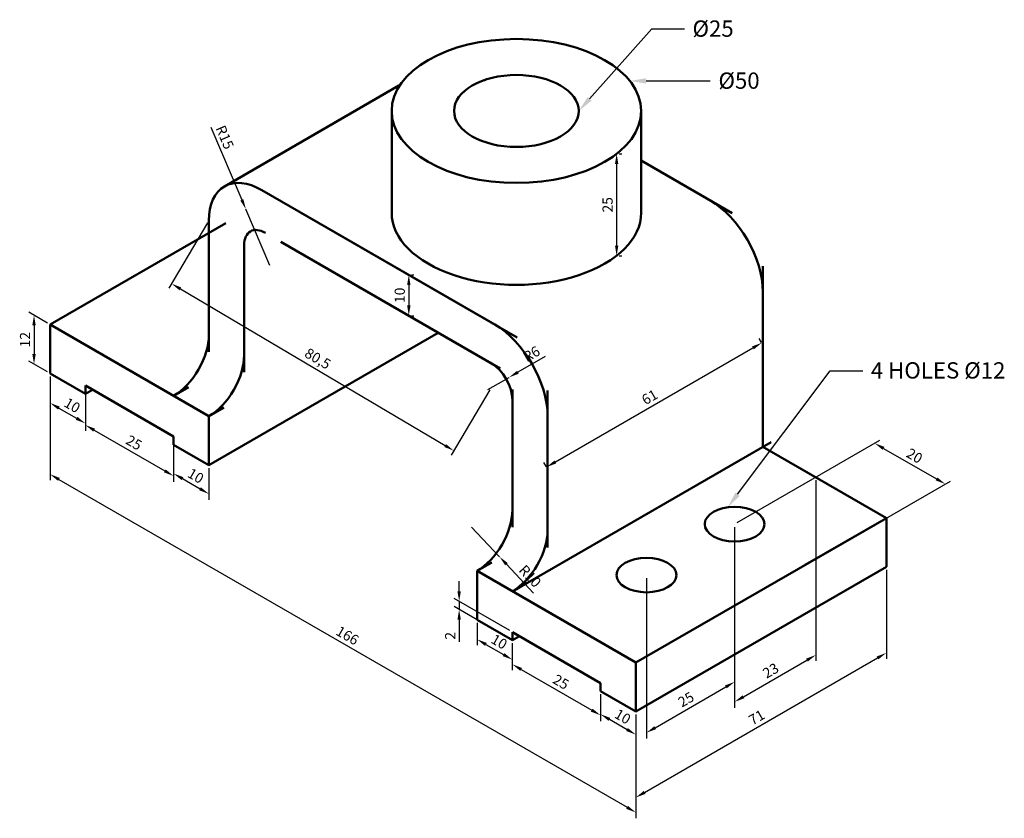
# Model space of a CAD drawing. Units: millimetres. Extents: x 2147 to 2389, y 1166 to 1362.
import ezdxf
from ezdxf import colors
from ezdxf.entities.mleader import LeaderData, LeaderLine
from ezdxf.math import Vec2, Vec3

# ---------------------------------------------------------------- set-up
doc = ezdxf.new("R2010")
doc.units = ezdxf.units.MM
for name, color, linetype, lineweight in [('M-DIMS', 2, 'Continuous', 25), ('M-OUTL', 7, 'Continuous', 50), ('M-TEXT', 3, 'Continuous', 25)]:
    doc.layers.add(name, color=color, linetype=linetype, lineweight=lineweight)
doc.styles.get("Standard").update_dxf_attribs({"font": 'arial.ttf'})
doc.dimstyles.new('ISO-25', dxfattribs={"dimtxt": 2.5, "dimasz": 2.5, "dimexe": 1.25, "dimexo": 0.625, "dimtad": 1, "dimtxsty": 'Standard', "dimcen": 2.5, "dimadec": 0, "dimazin": 0, "dimtfac": 1, "dimtmove": 0, "dimatfit": 3, "dimfxl": 1, "dimarcsym": 0})

# ---------------------------------------------------------------- blocks, each defined once
blk = doc.blocks.new('*D1')
at = {"layer": 'Defpoints', "color": 0, "transparency": 16777216}
for p in [(2154.59, 1274.83), (2298.35, 1191.83), (2298.35, 1167.06)]:
    blk.add_point(p, dxfattribs=at)
at = {"layer": 'M-DIMS', "color": 0, "lineweight": -2, "transparency": 16777216}
for p, q in [((2154.59, 1274.1), (2154.59, 1248.61)), ((2156.76, 1248.81), (2296.19, 1168.31)), ((2298.35, 1191.1), (2298.35, 1165.61))]:
    blk.add_line(p, q, dxfattribs=at)
at = {"layer": 'M-DIMS', "color": 0, "transparency": 16777216}
for points in [[(2156.97, 1249.17), (2156.55, 1248.44), (2154.59, 1250.06)], [(2296.4, 1168.67), (2295.98, 1167.94), (2298.35, 1167.06)]]:
    blk.add_solid(points, dxfattribs=at)
at = {"layer": 'M-DIMS', "color": 0, "transparency": 16777216, "insert": (2227.42, 1210.2), "char_height": 2.5, "attachment_point": 5, "rotation": 330}
blk.add_mtext('166', dxfattribs=at)
blk = doc.blocks.new('*D2')
at = {"layer": 'Defpoints', "color": 0, "transparency": 16777216}
for p in [(2154.59, 1274.83), (2163.25, 1269.83), (2163.25, 1262.56)]:
    blk.add_point(p, dxfattribs=at)
at = {"layer": 'M-DIMS', "color": 0, "lineweight": -2, "transparency": 16777216}
for p, q in [((2154.59, 1274.1), (2154.59, 1266.12)), ((2163.25, 1269.1), (2163.25, 1261.12)), ((2156.76, 1266.31), (2161.09, 1263.81))]:
    blk.add_line(p, q, dxfattribs=at)
at = {"layer": 'M-DIMS', "color": 0, "transparency": 16777216}
for points in [[(2156.97, 1266.67), (2156.55, 1265.95), (2154.59, 1267.56)], [(2161.3, 1264.17), (2160.88, 1263.45), (2163.25, 1262.56)]]:
    blk.add_solid(points, dxfattribs=at)
at = {"layer": 'M-DIMS', "color": 0, "transparency": 16777216, "insert": (2159.87, 1266.71), "char_height": 2.5, "attachment_point": 5, "rotation": 330}
blk.add_mtext('10', dxfattribs=at)
blk = doc.blocks.new('*D3')
at = {"layer": 'Defpoints', "color": 0, "transparency": 16777216}
for p in [(2163.25, 1271.83), (2184.9, 1259.33), (2184.9, 1249.65)]:
    blk.add_point(p, dxfattribs=at)
at = {"layer": 'M-DIMS', "color": 0, "lineweight": -2, "transparency": 16777216}
for p, q in [((2163.25, 1271.1), (2163.25, 1260.71)), ((2165.42, 1260.9), (2182.74, 1250.9)), ((2184.9, 1258.6), (2184.9, 1248.21))]:
    blk.add_line(p, q, dxfattribs=at)
at = {"layer": 'M-DIMS', "color": 0, "transparency": 16777216}
for points in [[(2165.63, 1261.26), (2165.21, 1260.54), (2163.25, 1262.15)], [(2182.95, 1251.26), (2182.53, 1250.54), (2184.9, 1249.65)]]:
    blk.add_solid(points, dxfattribs=at)
at = {"layer": 'M-DIMS', "color": 0, "transparency": 16777216, "insert": (2175.03, 1257.55), "char_height": 2.5, "attachment_point": 5, "rotation": 330}
blk.add_mtext('25', dxfattribs=at)
blk = doc.blocks.new('*D4')
at = {"layer": 'Defpoints', "color": 0, "transparency": 16777216}
for p in [(2184.9, 1257.33), (2193.56, 1252.33), (2193.56, 1245.25)]:
    blk.add_point(p, dxfattribs=at)
at = {"layer": 'M-DIMS', "color": 0, "lineweight": -2, "transparency": 16777216}
for p, q in [((2184.9, 1256.6), (2184.9, 1248.81)), ((2193.56, 1251.6), (2193.56, 1243.81)), ((2187.07, 1249), (2191.4, 1246.5))]:
    blk.add_line(p, q, dxfattribs=at)
at = {"layer": 'M-DIMS', "color": 0, "transparency": 16777216}
for points in [[(2187.28, 1249.36), (2186.86, 1248.64), (2184.9, 1250.25)], [(2191.61, 1246.86), (2191.19, 1246.14), (2193.56, 1245.25)]]:
    blk.add_solid(points, dxfattribs=at)
at = {"layer": 'M-DIMS', "color": 0, "transparency": 16777216, "insert": (2190.18, 1249.4), "char_height": 2.5, "attachment_point": 5, "rotation": 330}
blk.add_mtext('10', dxfattribs=at)
blk = doc.blocks.new('*D5')
at = {"layer": 'Defpoints', "color": 0, "transparency": 16777216}
for p in [(2154.59, 1286.83), (2150.65, 1277.1), (2154.59, 1274.83)]:
    blk.add_point(p, dxfattribs=at)
at = {"layer": 'M-DIMS', "color": 0, "lineweight": -2, "transparency": 16777216}
for p, q in [((2153.97, 1287.19), (2149.4, 1289.82)), ((2150.65, 1286.6), (2150.65, 1279.6)), ((2153.97, 1275.19), (2149.4, 1277.82))]:
    blk.add_line(p, q, dxfattribs=at)
at = {"layer": 'M-DIMS', "color": 0, "transparency": 16777216}
for points in [[(2150.23, 1286.6), (2151.07, 1286.6), (2150.65, 1289.1)], [(2150.23, 1279.6), (2151.07, 1279.6), (2150.65, 1277.1)]]:
    blk.add_solid(points, dxfattribs=at)
at = {"layer": 'M-DIMS', "color": 0, "transparency": 16777216, "insert": (2148.77, 1283.1), "char_height": 2.5, "attachment_point": 5, "rotation": 90}
blk.add_mtext('12', dxfattribs=at)
blk = doc.blocks.new('*D6')
at = {"layer": 'Defpoints', "color": 0, "transparency": 16777216}
for p in [(2259.38, 1214.33), (2268.04, 1209.33), (2268.04, 1204.55)]:
    blk.add_point(p, dxfattribs=at)
at = {"layer": 'M-DIMS', "color": 0, "lineweight": -2, "transparency": 16777216}
for p, q in [((2259.38, 1213.6), (2259.38, 1208.1)), ((2268.04, 1208.6), (2268.04, 1203.1)), ((2261.55, 1208.3), (2265.88, 1205.8))]:
    blk.add_line(p, q, dxfattribs=at)
at = {"layer": 'M-DIMS', "color": 0, "transparency": 16777216}
for points in [[(2261.76, 1208.66), (2261.34, 1207.94), (2259.38, 1209.55)], [(2266.09, 1206.16), (2265.67, 1205.44), (2268.04, 1204.55)]]:
    blk.add_solid(points, dxfattribs=at)
at = {"layer": 'M-DIMS', "color": 0, "transparency": 16777216, "insert": (2264.66, 1208.69), "char_height": 2.5, "attachment_point": 5, "rotation": 330}
blk.add_mtext('10', dxfattribs=at)
blk = doc.blocks.new('*D7')
at = {"layer": 'Defpoints', "color": 0, "transparency": 16777216}
for p in [(2254.99, 1216.86), (2268.04, 1211.33), (2268.04, 1209.33)]:
    blk.add_point(p, dxfattribs=at)
at = {"layer": 'M-DIMS', "color": 0, "lineweight": -2, "transparency": 16777216}
for p, q in [((2254.99, 1221.36), (2254.99, 1223.86)), ((2267.42, 1211.69), (2253.74, 1219.59)), ((2254.99, 1218.86), (2254.99, 1216.86)), ((2267.42, 1209.69), (2253.74, 1217.59)), ((2254.99, 1214.36), (2254.99, 1208.96))]:
    blk.add_line(p, q, dxfattribs=at)
at = {"layer": 'M-DIMS', "color": 0, "transparency": 16777216}
for points in [[(2254.57, 1221.36), (2255.4, 1221.36), (2254.99, 1218.86)], [(2254.57, 1214.36), (2255.4, 1214.36), (2254.99, 1216.86)]]:
    blk.add_solid(points, dxfattribs=at)
at = {"layer": 'M-DIMS', "color": 0, "transparency": 16777216, "insert": (2253.11, 1210.41), "char_height": 2.5, "attachment_point": 5, "rotation": 90}
blk.add_mtext('2', dxfattribs=at)
blk = doc.blocks.new('*D8')
at = {"layer": 'Defpoints', "color": 0, "transparency": 16777216}
for p in [(2268.04, 1209.33), (2289.69, 1196.83), (2289.69, 1190.91)]:
    blk.add_point(p, dxfattribs=at)
at = {"layer": 'M-DIMS', "color": 0, "lineweight": -2, "transparency": 16777216}
for p, q in [((2268.04, 1208.6), (2268.04, 1201.97)), ((2270.21, 1202.16), (2287.53, 1192.16)), ((2289.69, 1196.1), (2289.69, 1189.47))]:
    blk.add_line(p, q, dxfattribs=at)
at = {"layer": 'M-DIMS', "color": 0, "transparency": 16777216}
for points in [[(2270.42, 1202.52), (2270, 1201.8), (2268.04, 1203.41)], [(2287.74, 1192.52), (2287.32, 1191.8), (2289.69, 1190.91)]]:
    blk.add_solid(points, dxfattribs=at)
at = {"layer": 'M-DIMS', "color": 0, "transparency": 16777216, "insert": (2279.82, 1198.81), "char_height": 2.5, "attachment_point": 5, "rotation": 330}
blk.add_mtext('25', dxfattribs=at)
blk = doc.blocks.new('*D9')
at = {"layer": 'Defpoints', "color": 0, "transparency": 16777216}
for p in [(2289.69, 1196.83), (2298.35, 1191.83), (2298.35, 1186.16)]:
    blk.add_point(p, dxfattribs=at)
at = {"layer": 'M-DIMS', "color": 0, "lineweight": -2, "transparency": 16777216}
for p, q in [((2289.69, 1196.1), (2289.69, 1189.72)), ((2291.86, 1189.91), (2296.19, 1187.41)), ((2298.35, 1191.1), (2298.35, 1184.72))]:
    blk.add_line(p, q, dxfattribs=at)
at = {"layer": 'M-DIMS', "color": 0, "transparency": 16777216}
for points in [[(2292.07, 1190.27), (2291.65, 1189.55), (2289.69, 1191.16)], [(2296.4, 1187.77), (2295.98, 1187.05), (2298.35, 1186.16)]]:
    blk.add_solid(points, dxfattribs=at)
at = {"layer": 'M-DIMS', "color": 0, "transparency": 16777216, "insert": (2294.97, 1190.31), "char_height": 2.5, "attachment_point": 5, "rotation": 330}
blk.add_mtext('10', dxfattribs=at)
blk = doc.blocks.new('*D10')
at = {"layer": 'Defpoints', "color": 0, "transparency": 16777216}
for p in [(2359.84, 1227.33), (2359.84, 1206.23), (2298.35, 1191.83)]:
    blk.add_point(p, dxfattribs=at)
at = {"layer": 'M-DIMS', "color": 0, "lineweight": -2, "transparency": 16777216}
for p, q in [((2359.84, 1226.6), (2359.84, 1204.79)), ((2300.52, 1171.98), (2357.68, 1204.98)), ((2298.35, 1191.1), (2298.35, 1169.29))]:
    blk.add_line(p, q, dxfattribs=at)
at = {"layer": 'M-DIMS', "color": 0, "transparency": 16777216}
for points in [[(2357.47, 1205.34), (2357.88, 1204.62), (2359.84, 1206.23)], [(2300.31, 1172.34), (2300.73, 1171.62), (2298.35, 1170.73)]]:
    blk.add_solid(points, dxfattribs=at)
at = {"layer": 'M-DIMS', "color": 0, "transparency": 16777216, "insert": (2328.16, 1190.11), "char_height": 2.5, "attachment_point": 5, "rotation": 30}
blk.add_mtext('71', dxfattribs=at)
blk = doc.blocks.new('*D11')
at = {"layer": 'Defpoints', "color": 0, "transparency": 16777216}
for p in [(2322.6, 1237.83), (2300.95, 1225.33), (2322.6, 1199.11)]:
    blk.add_point(p, dxfattribs=at)
at = {"layer": 'M-DIMS', "color": 0, "lineweight": -2, "transparency": 16777216}
for p, q in [((2322.6, 1237.1), (2322.6, 1197.67)), ((2300.95, 1224.6), (2300.95, 1185.17)), ((2303.12, 1187.86), (2320.44, 1197.86))]:
    blk.add_line(p, q, dxfattribs=at)
at = {"layer": 'M-DIMS', "color": 0, "transparency": 16777216}
for points in [[(2320.23, 1198.22), (2320.65, 1197.5), (2322.6, 1199.11)], [(2302.91, 1188.22), (2303.32, 1187.5), (2300.95, 1186.61)]]:
    blk.add_solid(points, dxfattribs=at)
at = {"layer": 'M-DIMS', "color": 0, "transparency": 16777216, "insert": (2310.83, 1194.51), "char_height": 2.5, "attachment_point": 5, "rotation": 30}
blk.add_mtext('25', dxfattribs=at)
blk = doc.blocks.new('*D12')
at = {"layer": 'Defpoints', "color": 0, "transparency": 16777216}
for p in [(2374.31, 1247.68), (2322.6, 1237.83), (2339.92, 1227.83)]:
    blk.add_point(p, dxfattribs=at)
at = {"layer": 'M-DIMS', "color": 0, "lineweight": -2, "transparency": 16777216}
for p, q in [((2323.23, 1238.19), (2358.23, 1258.4)), ((2359.15, 1256.43), (2372.14, 1248.93)), ((2340.55, 1228.19), (2375.56, 1248.4))]:
    blk.add_line(p, q, dxfattribs=at)
at = {"layer": 'M-DIMS', "color": 0, "transparency": 16777216}
for points in [[(2359.36, 1256.79), (2358.94, 1256.07), (2356.98, 1257.68)], [(2372.35, 1249.29), (2371.93, 1248.57), (2374.31, 1247.68)]]:
    blk.add_solid(points, dxfattribs=at)
at = {"layer": 'M-DIMS', "color": 0, "transparency": 16777216, "insert": (2366.6, 1254.32), "char_height": 2.5, "attachment_point": 5, "rotation": 330}
blk.add_mtext('20', dxfattribs=at)
blk = doc.blocks.new('*D13')
at = {"layer": 'Defpoints', "color": 0, "transparency": 16777216}
for p in [(2242.63, 1299), (2242.63, 1289), (2242.63, 1289)]:
    blk.add_point(p, dxfattribs=at)
at = {"layer": 'M-DIMS', "color": 0, "lineweight": -2, "transparency": 16777216}
for p, q in [((2243.26, 1299), (2243.88, 1299)), ((2242.63, 1296.5), (2242.63, 1291.5)), ((2243.26, 1289), (2243.88, 1289))]:
    blk.add_line(p, q, dxfattribs=at)
at = {"layer": 'M-DIMS', "color": 0, "transparency": 16777216}
for points in [[(2242.22, 1296.5), (2243.05, 1296.5), (2242.63, 1299)], [(2242.22, 1291.5), (2243.05, 1291.5), (2242.63, 1289)]]:
    blk.add_solid(points, dxfattribs=at)
at = {"layer": 'M-DIMS', "color": 0, "transparency": 16777216, "insert": (2240.73, 1294), "char_height": 2.5, "attachment_point": 5, "rotation": 90}
blk.add_mtext('10', dxfattribs=at)
blk = doc.blocks.new('*D14')
at = {"layer": 'Defpoints', "color": 0, "transparency": 16777216}
for p in [(2293.64, 1328.72), (2293.64, 1303.72), (2293.64, 1303.72)]:
    blk.add_point(p, dxfattribs=at)
at = {"layer": 'M-DIMS', "color": 0, "lineweight": -2, "transparency": 16777216}
for p, q in [((2294.27, 1328.72), (2294.89, 1328.72)), ((2293.64, 1326.22), (2293.64, 1306.22)), ((2294.27, 1303.72), (2294.89, 1303.72))]:
    blk.add_line(p, q, dxfattribs=at)
at = {"layer": 'M-DIMS', "color": 0, "transparency": 16777216}
for points in [[(2293.23, 1326.22), (2294.06, 1326.22), (2293.64, 1328.72)], [(2293.23, 1306.22), (2294.06, 1306.22), (2293.64, 1303.72)]]:
    blk.add_solid(points, dxfattribs=at)
at = {"layer": 'M-DIMS', "color": 0, "transparency": 16777216, "insert": (2291.74, 1316.22), "char_height": 2.5, "attachment_point": 5, "rotation": 90}
blk.add_mtext('25', dxfattribs=at)
blk = doc.blocks.new('*D15')
at = {"layer": 'Defpoints', "color": 0, "transparency": 16777216}
for p in [(2342.52, 1249.33), (2322.6, 1237.83), (2342.52, 1205.7)]:
    blk.add_point(p, dxfattribs=at)
at = {"layer": 'M-DIMS', "color": 0, "lineweight": -2, "transparency": 16777216}
for p, q in [((2342.52, 1248.6), (2342.52, 1204.25)), ((2322.6, 1237.1), (2322.6, 1192.75)), ((2324.77, 1195.45), (2340.36, 1204.45))]:
    blk.add_line(p, q, dxfattribs=at)
at = {"layer": 'M-DIMS', "color": 0, "transparency": 16777216}
for points in [[(2340.15, 1204.81), (2340.56, 1204.08), (2342.52, 1205.7)], [(2324.56, 1195.81), (2324.98, 1195.08), (2322.6, 1194.2)]]:
    blk.add_solid(points, dxfattribs=at)
at = {"layer": 'M-DIMS', "color": 0, "transparency": 16777216, "insert": (2331.61, 1201.59), "char_height": 2.5, "attachment_point": 5, "rotation": 30}
blk.add_mtext('23', dxfattribs=at)
blk = doc.blocks.new('*D16')
at = {"layer": 'Defpoints', "color": 0, "transparency": 16777216}
for p in [(2329.27, 1282.34), (2329.53, 1281.88), (2276.7, 1251.38)]:
    blk.add_point(p, dxfattribs=at)
at = {"layer": 'M-DIMS', "color": 0, "lineweight": -2, "transparency": 16777216}
for p, q in [((2329.22, 1282.42), (2328.64, 1283.42)), ((2278.6, 1253.09), (2327.1, 1281.09)), ((2276.39, 1251.92), (2275.81, 1252.92))]:
    blk.add_line(p, q, dxfattribs=at)
at = {"layer": 'M-DIMS', "color": 0, "transparency": 16777216}
for points in [[(2326.89, 1281.45), (2327.31, 1280.73), (2329.27, 1282.34)], [(2278.4, 1253.45), (2278.81, 1252.73), (2276.44, 1251.84)]]:
    blk.add_solid(points, dxfattribs=at)
at = {"layer": 'M-DIMS', "color": 0, "transparency": 16777216, "insert": (2301.9, 1268.73), "char_height": 2.5, "attachment_point": 5, "rotation": 30}
blk.add_mtext('61', dxfattribs=at)
blk = doc.blocks.new('*D17')
at = {"layer": 'Defpoints', "color": 0, "transparency": 16777216}
for p in [(2258.04, 1237.1), (2264.89, 1229.81)]:
    blk.add_point(p, dxfattribs=at)
at = {"layer": 'M-DIMS', "color": 0, "lineweight": -2, "transparency": 16777216}
for p, q in [((2258.04, 1237.1), (2264.89, 1229.81)), ((2273.26, 1220.91), (2266.6, 1227.99))]:
    blk.add_line(p, q, dxfattribs=at)
at = {"layer": 'M-DIMS', "color": 0, "transparency": 16777216}
blk.add_solid([(2266.91, 1228.28), (2266.3, 1227.71), (2264.89, 1229.81)], dxfattribs=at)
at = {"layer": 'M-DIMS', "color": 0, "transparency": 16777216, "insert": (2272.17, 1224.84), "char_height": 2.5, "attachment_point": 5, "rotation": 313.232}
blk.add_mtext('R10', dxfattribs=at)
blk = doc.blocks.new('*D18')
at = {"layer": 'Defpoints', "color": 0, "transparency": 16777216}
for p in [(2202.64, 1315.13), (2208.56, 1301.35)]:
    blk.add_point(p, dxfattribs=at)
at = {"layer": 'M-DIMS', "color": 0, "lineweight": -2, "transparency": 16777216}
for p, q in [((2194.01, 1335.24), (2201.66, 1317.42)), ((2208.56, 1301.35), (2202.64, 1315.13))]:
    blk.add_line(p, q, dxfattribs=at)
at = {"layer": 'M-DIMS', "color": 0, "transparency": 16777216}
blk.add_solid([(2202.04, 1317.59), (2201.28, 1317.26), (2202.64, 1315.13)], dxfattribs=at)
at = {"layer": 'M-DIMS', "color": 0, "transparency": 16777216, "insert": (2197.18, 1332.66), "char_height": 2.5, "attachment_point": 5, "rotation": 293.2425}
blk.add_mtext('R15', dxfattribs=at)
blk = doc.blocks.new('*D19')
at = {"layer": 'Defpoints', "color": 0, "transparency": 16777216}
for p in [(2267.24, 1273.86), (2262.04, 1270.86)]:
    blk.add_point(p, dxfattribs=at)
at = {"layer": 'M-DIMS', "color": 0, "lineweight": -2, "transparency": 16777216}
for p, q in [((2276.14, 1279), (2269.4, 1275.11)), ((2262.04, 1270.86), (2267.24, 1273.86))]:
    blk.add_line(p, q, dxfattribs=at)
at = {"layer": 'M-DIMS', "color": 0, "transparency": 16777216}
blk.add_solid([(2269.2, 1275.47), (2269.61, 1274.75), (2267.24, 1273.86)], dxfattribs=at)
at = {"layer": 'M-DIMS', "color": 0, "transparency": 16777216, "insert": (2272.9, 1279.33), "char_height": 2.5, "attachment_point": 5, "rotation": 30}
blk.add_mtext('R6', dxfattribs=at)
blk = doc.blocks.new('*D20')
at = {"layer": 'Defpoints', "color": 0, "transparency": 16777216}
for p in [(2193.57, 1312.33), (2262.85, 1271.33), (2253.69, 1255.85)]:
    blk.add_point(p, dxfattribs=at)
at = {"layer": 'M-DIMS', "color": 0, "lineweight": -2, "transparency": 16777216}
for p, q in [((2193.25, 1311.79), (2183.77, 1295.78)), ((2186.56, 1295.58), (2251.54, 1257.13)), ((2262.53, 1270.79), (2253.05, 1254.78))]:
    blk.add_line(p, q, dxfattribs=at)
at = {"layer": 'M-DIMS', "color": 0, "transparency": 16777216}
for points in [[(2186.77, 1295.94), (2186.35, 1295.22), (2184.41, 1296.85)], [(2251.75, 1257.48), (2251.33, 1256.77), (2253.69, 1255.85)]]:
    blk.add_solid(points, dxfattribs=at)
at = {"layer": 'M-DIMS', "color": 0, "transparency": 16777216, "insert": (2220.13, 1278.18), "char_height": 2.5, "attachment_point": 5, "rotation": 329.3836}
blk.add_mtext('80,5', dxfattribs=at)

msp = doc.modelspace()

# ---------------------------------------------------------------- linework, layer by layer
at = {"layer": 'M-OUTL'}
for p, q in [((2261.392, 1346.845), (2261.612, 1346.972)), ((2197.37, 1320.736), (2240.193, 1345.46)), ((2238.429, 1339.246), (2238.429, 1314.246)), ((2299.666, 1339.246), (2299.666, 1314.246)), ((2322.03, 1314.156), (2299.666, 1327.068)), ((2263.713, 1286.826), (2206.556, 1319.826)), ((2193.565, 1312.326), (2193.565, 1284.326)), ((2269.203, 1283.656), (2216.064, 1314.336)), ((2154.593, 1286.826), (2197.756, 1311.746)), ((2202.225, 1279.326), (2202.225, 1306.326)), ((2265.042, 1276.058), (2211.225, 1307.13)), ((2193.564, 1280.099), (2193.564, 1301.345)), ((2202.225, 1275.099), (2202.225, 1301.934)), ((2329.53, 1265.486), (2329.53, 1301.166)), ((2329.531, 1294.826), (2329.531, 1256.826)), ((2154.593, 1274.826), (2154.593, 1286.826)), ((2193.564, 1264.326), (2154.593, 1286.826)), ((2154.593, 1286.826), (2154.593, 1274.826)), ((2193.564, 1252.326), (2249.856, 1284.826)), ((2154.593, 1274.826), (2163.253, 1269.826)), ((2163.253, 1269.826), (2163.253, 1271.826)), ((2163.253, 1271.826), (2184.904, 1259.326)), ((2188.564, 1271.439), (2184.904, 1269.326)), ((2163.254, 1269.826), (2164.986, 1270.826)), ((2268.042, 1237.099), (2268.042, 1270.862)), ((2276.703, 1232.099), (2276.703, 1270.666)), ((2193.564, 1264.326), (2197.225, 1266.439)), ((2193.564, 1264.326), (2193.564, 1252.326)), ((2184.904, 1259.326), (2184.904, 1257.326)), ((2184.904, 1257.326), (2193.564, 1252.326)), ((2268.042, 1221.326), (2331.54, 1257.986)), ((2359.842, 1239.326), (2329.531, 1256.826)), ((2337.03, 1252.496), (2359.841, 1239.326)), ((2359.841, 1239.326), (2298.353, 1203.826)), ((2359.841, 1239.326), (2339.923, 1227.826)), ((2359.841, 1227.326), (2359.841, 1239.326)), ((2259.382, 1226.326), (2263.042, 1228.439)), ((2298.353, 1203.826), (2259.382, 1226.326)), ((2259.382, 1226.326), (2259.382, 1214.326)), ((2298.353, 1191.826), (2359.841, 1227.326)), ((2271.703, 1223.439), (2268.042, 1221.326)), ((2259.382, 1214.326), (2268.042, 1209.326)), ((2268.042, 1209.326), (2268.042, 1211.326)), ((2268.042, 1211.326), (2289.693, 1198.826)), ((2268.043, 1209.326), (2269.775, 1210.326)), ((2298.353, 1203.826), (2298.353, 1191.826)), ((2289.693, 1198.826), (2289.693, 1196.826)), ((2289.693, 1196.826), (2298.353, 1191.826))]:
    msp.add_line(p, q, dxfattribs=at)
msp.add_arc((2261.392, 1331.845), 15, 90, 90.63178, dxfattribs=at)
for centre, major_axis in [((2269.047, 1339.246), (-30.619, 0)), ((2269.047, 1339.246), (-15.309, 0)), ((2322.602, 1237.826), (-7.348, 0)), ((2300.951, 1225.326), (-7.348, 0))]:
    msp.add_ellipse(centre, major_axis=major_axis, ratio=0.5773503, dxfattribs=at)
for centre, major_axis, start_param, end_param in [((2206.556, 1304.826), (-9.186, 15.91), 5.4977871, 6.2831853), ((2206.556, 1304.826), (-9.186, 15.91), 0, 0.7853982), ((2316.541, 1302.326), (-9.186, 15.91), 3.9269908, 5.4977871), ((2269.047, 1314.246), (-30.619, 0), 6.2831853, 9.424778), ((2207.422, 1303.326), (-3.674, 6.364), 5.4977871, 6.2831853), ((2207.422, 1303.326), (-3.674, 6.364), 0, 0.7853982), ((2263.713, 1271.826), (-9.186, 15.91), 3.9269908, 5.4977871), ((2184.905, 1279.326), (6.124, 10.606), 3.9269798, 5.4977981), ((2193.565, 1274.326), (6.124, 10.606), 3.9269798, 5.4977981), ((2262.847, 1271.326), (-3.674, 6.364), 3.9269908, 5.4977871), ((2259.383, 1236.326), (6.124, 10.606), 3.9269798, 5.4977981), ((2268.043, 1231.326), (6.124, 10.606), 3.9269798, 5.4977981)]:
    msp.add_ellipse(centre, major_axis=major_axis, ratio=0.5773503, start_param=start_param, end_param=end_param, dxfattribs=at)

# ---------------------------------------------------------------- dimensions: what is measured, and where the dimension line sits
at = {"layer": 'M-DIMS'}
dim = msp.add_radius_dim(center=(2208.564, 1301.345), mpoint=(2202.645, 1315.128), dimstyle='ISO-25', override={"dimclrd": 0, "dimclre": 0, "dimclrt": 0}, dxfattribs=at)
dim.commit()
dim.dimension.update_dxf_attribs({"geometry": '*D18', "text_midpoint": (2195.437, 1331.911), "dimtype": 164})
for base, p1, p2, angle, override, picture, middle in [((2293.643, 1303.717), (2293.643, 1328.717), (2293.643, 1303.717), 90, {"dimclrd": 0, "dimclre": 0, "dimclrt": 0}, '*D14', (2291.742, 1316.217)), ((2253.691, 1255.853), (2193.565, 1312.326), (2262.847, 1271.326), 329.38363, {"dimrnd": 0}, '*D20', (2220.133, 1278.184)), ((2242.633, 1288.996), (2242.633, 1298.996), (2242.633, 1288.996), 90, {"dimclrd": 0, "dimclre": 0, "dimclrt": 0}, '*D13', (2240.732, 1293.996)), ((2150.65, 1277.102), (2154.593, 1286.826), (2154.593, 1274.826), 90, {"dimclrd": 0, "dimclre": 0, "dimclrt": 0}, '*D5', (2148.77, 1283.102)), ((2254.987, 1216.863), (2268.042, 1211.326), (2268.042, 1209.326), 90, {"dimclrd": 0, "dimclre": 0, "dimclrt": 0}, '*D7', (2253.107, 1210.411))]:
    dim = msp.add_linear_dim(base=base, p1=p1, p2=p2, angle=angle, dimstyle='ISO-25', override=override, dxfattribs=at)
    dim.commit()
    dim.dimension.update_dxf_attribs({"geometry": picture, "text_midpoint": middle})
for p1, p2, distance, picture, middle in [((2276.703, 1251.383), (2329.53, 1281.883), 0.526, '*D16', (2301.903, 1268.735)), ((2154.593, 1274.826), (2298.353, 1191.826), -21.452, '*D1', (2227.424, 1210.202)), ((2154.593, 1274.826), (2163.253, 1269.826), -6.29, '*D2', (2159.874, 1266.71)), ((2163.253, 1271.826), (2184.904, 1259.326), -8.379, '*D3', (2175.029, 1257.547)), ((2184.904, 1257.326), (2193.564, 1252.326), -6.128, '*D4', (2190.185, 1249.397)), ((2322.602, 1237.826), (2339.923, 1227.826), 34.383, '*D12', (2366.596, 1254.324)), ((2322.602, 1237.826), (2342.521, 1249.326), -37.785, '*D15', (2331.61, 1201.593)), ((2300.951, 1225.326), (2322.602, 1237.826), -33.527, '*D11', (2310.826, 1194.508)), ((2298.353, 1191.826), (2359.841, 1227.326), -18.269, '*D10', (2328.157, 1190.109)), ((2259.382, 1214.326), (2268.042, 1209.326), -4.139, '*D6', (2264.663, 1208.693)), ((2268.042, 1209.326), (2289.693, 1196.826), -5.123, '*D8', (2279.818, 1198.807)), ((2289.693, 1196.826), (2298.353, 1191.826), -4.903, '*D9', (2294.974, 1190.311))]:
    dim = msp.add_aligned_dim(p1=p1, p2=p2, distance=distance, dimstyle='ISO-25', override={"dimclrd": 0, "dimclre": 0, "dimclrt": 0}, dxfattribs=at)
    dim.commit()
    dim.dimension.update_dxf_attribs({"geometry": picture, "text_midpoint": middle})
for center, mpoint, picture, middle in [((2262.042, 1270.862), (2267.239, 1273.862), '*D19', (2272.904, 1279.328)), ((2258.042, 1237.099), (2264.892, 1229.814), '*D17', (2272.173, 1224.845))]:
    dim = msp.add_radius_dim(center=center, mpoint=mpoint, dimstyle='ISO-25', override={"dimclrd": 0, "dimclre": 0, "dimclrt": 0}, dxfattribs=at)
    dim.commit()
    dim.dimension.update_dxf_attribs({"geometry": picture, "text_midpoint": middle})

# ---------------------------------------------------------------- leaders
at = {"layer": 'M-TEXT'}
ml = msp.add_multileader_mtext('Standard', dxfattribs=at)
ml.set_content('%%C25', color=256)
ml.set_leader_properties()
ml.build(insert=Vec2(0, 0))
ctx = ml.context
ctx.base_point, ctx.plane_origin = Vec3(2310.261, 1359.39), Vec3(2284.357, 1339.246)
notes = []
notes.append((ctx, [(0, (1, 1, 0), (2302.261, 1359.39), (1, 0), 8, [(0, [(2284.357, 1339.246)], 0, [])])]))
ctx.mtext.insert, ctx.mtext.flow_direction = Vec3(2312.261, 1361.47), 5
ml = msp.add_multileader_mtext('Standard', dxfattribs=at)
ml.set_content('%%C50', color=256)
ml.set_leader_properties()
ml.build(insert=Vec2(0, 0))
ctx = ml.context
ctx.base_point, ctx.plane_origin = Vec3(2316.63, 1346.617), Vec3(2296.877, 1346.617)
notes.append((ctx, [(0, (1, 1, 0), (2308.63, 1346.617), (1, 0), 8, [(0, [(2296.877, 1346.617)], 0, [])])]))
ctx.mtext.insert, ctx.mtext.flow_direction = Vec3(2318.63, 1348.697), 5
ml = msp.add_multileader_mtext('Standard', dxfattribs=at)
ml.set_content('4 HOLES %%C12', color=256)
ml.set_leader_properties()
ml.build(insert=Vec2(0, 0))
ctx = ml.context
ctx.base_point, ctx.plane_origin = Vec3(2354.032, 1275.486), Vec3(2320.907, 1241.954)
notes.append((ctx, [(0, (1, 1, 0), (2346.032, 1275.486), (1, 0), 8, [(0, [(2320.907, 1241.954)], 0, [])])]))
ctx.mtext.insert, ctx.mtext.flow_direction = Vec3(2356.032, 1277.566), 5
for ctx, leaders in notes:
    for number, flags, end, landing, length, lines in leaders:
        leader = LeaderData()
        leader.index, (leader.has_last_leader_line, leader.has_dogleg_vector, leader.attachment_direction) = number, flags
        leader.last_leader_point, leader.dogleg_vector, leader.dogleg_length = Vec3(end), Vec3(landing), length
        for number, points, colour, breaks in lines:
            line = LeaderLine()
            line.index, line.vertices, line.color, line.breaks = number, Vec3.list(points), colors.encode_raw_color(colour), breaks
            leader.lines.append(line)
        ctx.leaders.append(leader)

doc.saveas('drawing.dxf')
